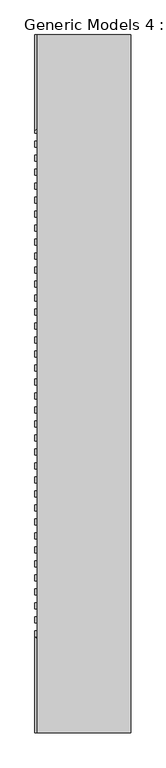
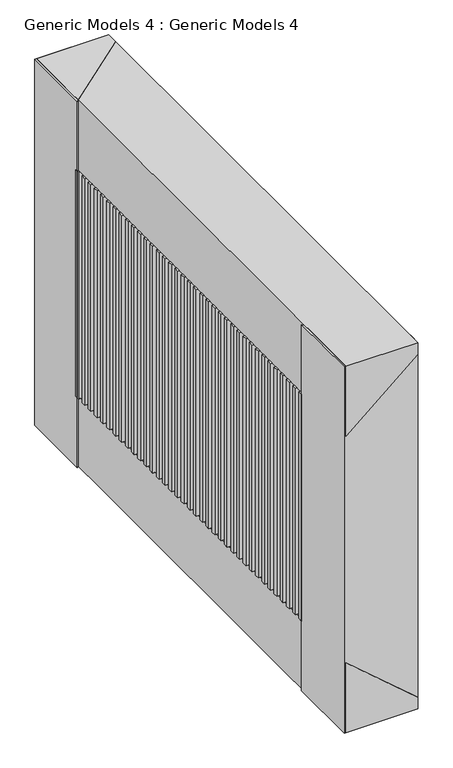
"""IFC4 building model written with IfcOpenShell, lengths in millimetres: proxy geometry, Generic Models 4 : Generic Models 4."""

from ifc_helpers import new_model, si_unit, frame, origin, place, context, project, spatial, polyline, outline, extrude, source, transform, mapped, element, save


def generic_models_4_generic_models_4_3dac0b09(model_context):
    return source(origin(), model_context, "Body", "SweptSolid", [
        extrude(outline(polyline([(7553.0590234, -3519.1296941), (7591.1590234, -3519.1296941), (7591.1590234, -3557.2296941), (7553.0590234, -3557.2296941), (7553.0590234, -3519.1296941)])), frame((0.0, 0.0, 4114.8), z_axis=(0.0, 0.0, 1.0), x_axis=(1.0, 0.0, 0.0)), (0.0, 0.0, 1.0), 1981.2),
        extrude(outline(polyline([(7553.0590234, -3430.2296941), (7591.1590234, -3430.2296941), (7591.1590234, -3468.3296941), (7553.0590234, -3468.3296941), (7553.0590234, -3430.2296941)])), frame((0.0, 0.0, 4114.8), z_axis=(0.0, 0.0, 1.0), x_axis=(1.0, 0.0, 0.0)), (0.0, 0.0, 1.0), 1981.2),
        extrude(outline(polyline([(7553.0590234, -3341.3296941), (7591.1590234, -3341.3296941), (7591.1590234, -3379.4296941), (7553.0590234, -3379.4296941), (7553.0590234, -3341.3296941)])), frame((0.0, 0.0, 4114.8), z_axis=(0.0, 0.0, 1.0), x_axis=(1.0, 0.0, 0.0)), (0.0, 0.0, 1.0), 1981.2),
        extrude(outline(polyline([(7553.0590234, -3252.4296941), (7591.1590234, -3252.4296941), (7591.1590234, -3290.5296941), (7553.0590234, -3290.5296941), (7553.0590234, -3252.4296941)])), frame((0.0, 0.0, 4114.8), z_axis=(0.0, 0.0, 1.0), x_axis=(1.0, 0.0, 0.0)), (0.0, 0.0, 1.0), 1981.2),
        extrude(outline(polyline([(7553.0590234, -3163.5296941), (7591.1590234, -3163.5296941), (7591.1590234, -3201.6296941), (7553.0590234, -3201.6296941), (7553.0590234, -3163.5296941)])), frame((0.0, 0.0, 4114.8), z_axis=(0.0, 0.0, 1.0), x_axis=(1.0, 0.0, 0.0)), (0.0, 0.0, 1.0), 1981.2),
        extrude(outline(polyline([(7553.0590234, -3074.6296941), (7591.1590234, -3074.6296941), (7591.1590234, -3112.7296941), (7553.0590234, -3112.7296941), (7553.0590234, -3074.6296941)])), frame((0.0, 0.0, 4114.8), z_axis=(0.0, 0.0, 1.0), x_axis=(1.0, 0.0, 0.0)), (0.0, 0.0, 1.0), 1981.2),
        extrude(outline(polyline([(7553.0590234, -2985.7296941), (7591.1590234, -2985.7296941), (7591.1590234, -3023.8296941), (7553.0590234, -3023.8296941), (7553.0590234, -2985.7296941)])), frame((0.0, 0.0, 4114.8), z_axis=(0.0, 0.0, 1.0), x_axis=(1.0, 0.0, 0.0)), (0.0, 0.0, 1.0), 1981.2),
        extrude(outline(polyline([(7553.0590234, -2896.8296941), (7591.1590234, -2896.8296941), (7591.1590234, -2934.9296941), (7553.0590234, -2934.9296941), (7553.0590234, -2896.8296941)])), frame((0.0, 0.0, 4114.8), z_axis=(0.0, 0.0, 1.0), x_axis=(1.0, 0.0, 0.0)), (0.0, 0.0, 1.0), 1981.2),
        extrude(outline(polyline([(7553.0590234, -2807.9296941), (7591.1590234, -2807.9296941), (7591.1590234, -2846.0296941), (7553.0590234, -2846.0296941), (7553.0590234, -2807.9296941)])), frame((0.0, 0.0, 4114.8), z_axis=(0.0, 0.0, 1.0), x_axis=(1.0, 0.0, 0.0)), (0.0, 0.0, 1.0), 1981.2),
        extrude(outline(polyline([(7553.0590234, -2719.0296941), (7591.1590234, -2719.0296941), (7591.1590234, -2757.1296941), (7553.0590234, -2757.1296941), (7553.0590234, -2719.0296941)])), frame((0.0, 0.0, 4114.8), z_axis=(0.0, 0.0, 1.0), x_axis=(1.0, 0.0, 0.0)), (0.0, 0.0, 1.0), 1981.2),
        extrude(outline(polyline([(7553.0590234, -2630.1296941), (7591.1590234, -2630.1296941), (7591.1590234, -2668.2296941), (7553.0590234, -2668.2296941), (7553.0590234, -2630.1296941)])), frame((0.0, 0.0, 4114.8), z_axis=(0.0, 0.0, 1.0), x_axis=(1.0, 0.0, 0.0)), (0.0, 0.0, 1.0), 1981.2),
        extrude(outline(polyline([(7553.0590234, -2541.2296941), (7591.1590234, -2541.2296941), (7591.1590234, -2579.3296941), (7553.0590234, -2579.3296941), (7553.0590234, -2541.2296941)])), frame((0.0, 0.0, 4114.8), z_axis=(0.0, 0.0, 1.0), x_axis=(1.0, 0.0, 0.0)), (0.0, 0.0, 1.0), 1981.2),
        extrude(outline(polyline([(7553.0590234, -2452.3296941), (7591.1590234, -2452.3296941), (7591.1590234, -2490.4296941), (7553.0590234, -2490.4296941), (7553.0590234, -2452.3296941)])), frame((0.0, 0.0, 4114.8), z_axis=(0.0, 0.0, 1.0), x_axis=(1.0, 0.0, 0.0)), (0.0, 0.0, 1.0), 1981.2),
        extrude(outline(polyline([(7553.0590234, -2363.4296941), (7591.1590234, -2363.4296941), (7591.1590234, -2401.5296941), (7553.0590234, -2401.5296941), (7553.0590234, -2363.4296941)])), frame((0.0, 0.0, 4114.8), z_axis=(0.0, 0.0, 1.0), x_axis=(1.0, 0.0, 0.0)), (0.0, 0.0, 1.0), 1981.2),
        extrude(outline(polyline([(7553.0590234, -2274.5296941), (7591.1590234, -2274.5296941), (7591.1590234, -2312.6296941), (7553.0590234, -2312.6296941), (7553.0590234, -2274.5296941)])), frame((0.0, 0.0, 4114.8), z_axis=(0.0, 0.0, 1.0), x_axis=(1.0, 0.0, 0.0)), (0.0, 0.0, 1.0), 1981.2),
        extrude(outline(polyline([(7553.0590234, -2185.6296941), (7591.1590234, -2185.6296941), (7591.1590234, -2223.7296941), (7553.0590234, -2223.7296941), (7553.0590234, -2185.6296941)])), frame((0.0, 0.0, 4114.8), z_axis=(0.0, 0.0, 1.0), x_axis=(1.0, 0.0, 0.0)), (0.0, 0.0, 1.0), 1981.2),
        extrude(outline(polyline([(7553.0590234, -2096.7296941), (7591.1590234, -2096.7296941), (7591.1590234, -2134.8296941), (7553.0590234, -2134.8296941), (7553.0590234, -2096.7296941)])), frame((0.0, 0.0, 4114.8), z_axis=(0.0, 0.0, 1.0), x_axis=(1.0, 0.0, 0.0)), (0.0, 0.0, 1.0), 1981.2),
        extrude(outline(polyline([(7553.0590234, -2007.8296941), (7591.1590234, -2007.8296941), (7591.1590234, -2045.9296941), (7553.0590234, -2045.9296941), (7553.0590234, -2007.8296941)])), frame((0.0, 0.0, 4114.8), z_axis=(0.0, 0.0, 1.0), x_axis=(1.0, 0.0, 0.0)), (0.0, 0.0, 1.0), 1981.2),
        extrude(outline(polyline([(7553.0590234, -1918.9296941), (7591.1590234, -1918.9296941), (7591.1590234, -1957.0296941), (7553.0590234, -1957.0296941), (7553.0590234, -1918.9296941)])), frame((0.0, 0.0, 4114.8), z_axis=(0.0, 0.0, 1.0), x_axis=(1.0, 0.0, 0.0)), (0.0, 0.0, 1.0), 1981.2),
        extrude(outline(polyline([(7553.0590234, -1830.0296941), (7591.1590234, -1830.0296941), (7591.1590234, -1868.1296941), (7553.0590234, -1868.1296941), (7553.0590234, -1830.0296941)])), frame((0.0, 0.0, 4114.8), z_axis=(0.0, 0.0, 1.0), x_axis=(1.0, 0.0, 0.0)), (0.0, 0.0, 1.0), 1981.2),
        extrude(outline(polyline([(7553.0590234, -1741.1296941), (7591.1590234, -1741.1296941), (7591.1590234, -1779.2296941), (7553.0590234, -1779.2296941), (7553.0590234, -1741.1296941)])), frame((0.0, 0.0, 4114.8), z_axis=(0.0, 0.0, 1.0), x_axis=(1.0, 0.0, 0.0)), (0.0, 0.0, 1.0), 1981.2),
        extrude(outline(polyline([(7553.0590234, -1652.2296941), (7591.1590234, -1652.2296941), (7591.1590234, -1690.3296941), (7553.0590234, -1690.3296941), (7553.0590234, -1652.2296941)])), frame((0.0, 0.0, 4114.8), z_axis=(0.0, 0.0, 1.0), x_axis=(1.0, 0.0, 0.0)), (0.0, 0.0, 1.0), 1981.2),
        extrude(outline(polyline([(7553.0590234, -1563.3296941), (7591.1590234, -1563.3296941), (7591.1590234, -1601.4296941), (7553.0590234, -1601.4296941), (7553.0590234, -1563.3296941)])), frame((0.0, 0.0, 4114.8), z_axis=(0.0, 0.0, 1.0), x_axis=(1.0, 0.0, 0.0)), (0.0, 0.0, 1.0), 1981.2),
        extrude(outline(polyline([(7553.0590234, -1474.4296941), (7591.1590234, -1474.4296941), (7591.1590234, -1512.5296941), (7553.0590234, -1512.5296941), (7553.0590234, -1474.4296941)])), frame((0.0, 0.0, 4114.8), z_axis=(0.0, 0.0, 1.0), x_axis=(1.0, 0.0, 0.0)), (0.0, 0.0, 1.0), 1981.2),
        extrude(outline(polyline([(7553.0590234, -1385.5296941), (7591.1590234, -1385.5296941), (7591.1590234, -1423.6296941), (7553.0590234, -1423.6296941), (7553.0590234, -1385.5296941)])), frame((0.0, 0.0, 4114.8), z_axis=(0.0, 0.0, 1.0), x_axis=(1.0, 0.0, 0.0)), (0.0, 0.0, 1.0), 1981.2),
        extrude(outline(polyline([(7553.0590234, -1296.6296941), (7591.1590234, -1296.6296941), (7591.1590234, -1334.7296941), (7553.0590234, -1334.7296941), (7553.0590234, -1296.6296941)])), frame((0.0, 0.0, 4114.8), z_axis=(0.0, 0.0, 1.0), x_axis=(1.0, 0.0, 0.0)), (0.0, 0.0, 1.0), 1981.2),
        extrude(outline(polyline([(7553.0590234, -1207.7296941), (7591.1590234, -1207.7296941), (7591.1590234, -1245.8296941), (7553.0590234, -1245.8296941), (7553.0590234, -1207.7296941)])), frame((0.0, 0.0, 4114.8), z_axis=(0.0, 0.0, 1.0), x_axis=(1.0, 0.0, 0.0)), (0.0, 0.0, 1.0), 1981.2),
        extrude(outline(polyline([(7553.0590234, -1118.8296941), (7591.1590234, -1118.8296941), (7591.1590234, -1156.9296941), (7553.0590234, -1156.9296941), (7553.0590234, -1118.8296941)])), frame((0.0, 0.0, 4114.8), z_axis=(0.0, 0.0, 1.0), x_axis=(1.0, 0.0, 0.0)), (0.0, 0.0, 1.0), 1981.2),
        extrude(outline(polyline([(7553.0590234, -1029.9296941), (7591.1590234, -1029.9296941), (7591.1590234, -1068.0296941), (7553.0590234, -1068.0296941), (7553.0590234, -1029.9296941)])), frame((0.0, 0.0, 4114.8), z_axis=(0.0, 0.0, 1.0), x_axis=(1.0, 0.0, 0.0)), (0.0, 0.0, 1.0), 1981.2),
        extrude(outline(polyline([(7553.0590234, -941.0296941), (7591.1590234, -941.0296941), (7591.1590234, -979.1296941), (7553.0590234, -979.1296941), (7553.0590234, -941.0296941)])), frame((0.0, 0.0, 4114.8), z_axis=(0.0, 0.0, 1.0), x_axis=(1.0, 0.0, 0.0)), (0.0, 0.0, 1.0), 1981.2),
        extrude(outline(polyline([(7553.0590234, -852.1296941), (7591.1590234, -852.1296941), (7591.1590234, -890.2296941), (7553.0590234, -890.2296941), (7553.0590234, -852.1296941)])), frame((0.0, 0.0, 4114.8), z_axis=(0.0, 0.0, 1.0), x_axis=(1.0, 0.0, 0.0)), (0.0, 0.0, 1.0), 1981.2),
        extrude(outline(polyline([(7553.0590234, -763.2296941), (7591.1590234, -763.2296941), (7591.1590234, -801.3296941), (7553.0590234, -801.3296941), (7553.0590234, -763.2296941)])), frame((0.0, 0.0, 4114.8), z_axis=(0.0, 0.0, 1.0), x_axis=(1.0, 0.0, 0.0)), (0.0, 0.0, 1.0), 1981.2),
        extrude(outline(polyline([(7553.0590234, -674.3296941), (7591.1590234, -674.3296941), (7591.1590234, -712.4296941), (7553.0590234, -712.4296941), (7553.0590234, -674.3296941)])), frame((0.0, 0.0, 4114.8), z_axis=(0.0, 0.0, 1.0), x_axis=(1.0, 0.0, 0.0)), (0.0, 0.0, 1.0), 1981.2),
        extrude(outline(polyline([(7553.0590234, -585.4296941), (7591.1590234, -585.4296941), (7591.1590234, -623.5296941), (7553.0590234, -623.5296941), (7553.0590234, -585.4296941)])), frame((0.0, 0.0, 4114.8), z_axis=(0.0, 0.0, 1.0), x_axis=(1.0, 0.0, 0.0)), (0.0, 0.0, 1.0), 1981.2),
        extrude(outline(polyline([(7553.0590234, -496.5296941), (7591.1590234, -496.5296941), (7591.1590234, -534.6296941), (7553.0590234, -534.6296941), (7553.0590234, -496.5296941)])), frame((0.0, 0.0, 4114.8), z_axis=(0.0, 0.0, 1.0), x_axis=(1.0, 0.0, 0.0)), (0.0, 0.0, 1.0), 1981.2),
        extrude(outline(polyline([(7553.0590234, -407.6296941), (7591.1590234, -407.6296941), (7591.1590234, -445.7296941), (7553.0590234, -445.7296941), (7553.0590234, -407.6296941)])), frame((0.0, 0.0, 4114.8), z_axis=(0.0, 0.0, 1.0), x_axis=(1.0, 0.0, 0.0)), (0.0, 0.0, 1.0), 1981.2),
        extrude(outline(polyline([(7553.0590234, -318.7296941), (7591.1590234, -318.7296941), (7591.1590234, -356.8296941), (7553.0590234, -356.8296941), (7553.0590234, -318.7296941)])), frame((0.0, 0.0, 4114.8), z_axis=(0.0, 0.0, 1.0), x_axis=(1.0, 0.0, 0.0)), (0.0, 0.0, 1.0), 1981.2),
        extrude(outline(polyline([(3505.2, 8162.6590234), (3606.8, 8162.6590234), (4114.8, 7567.1057451), (3505.2, 7567.1057451), (3505.2, 8162.6590234)])), frame((0.0, -4166.8296941, 0.0), z_axis=(0.0, 1.0, 0.0), x_axis=(0.0, 0.0, 1.0)), (0.0, 0.0, 1.0), 4434.2439479),
        extrude(outline(polyline([(6705.6, 8162.6590234), (6705.6, 7567.1057451), (6096.0, 7567.1057451), (6604.0, 8162.6590234), (6705.6, 8162.6590234)])), frame((0.0, -4166.8296941, 0.0), z_axis=(0.0, 1.0, 0.0), x_axis=(0.0, 0.0, 1.0)), (0.0, 0.0, 1.0), 4434.2439479),
        extrude(outline(polyline([(7553.0590234, -3557.2296941), (8162.6590234, -4065.2296941), (8162.6590234, -4166.8296941), (7553.0590234, -4166.8296941), (7553.0590234, -3557.2296941)])), frame((0.0, 0.0, 3505.2), z_axis=(0.0, 0.0, 1.0), x_axis=(1.0, 0.0, 0.0)), (0.0, 0.0, 1.0), 3200.4),
        extrude(outline(polyline([(7553.0590234, -342.1857463), (7553.0590234, 267.4142537), (8162.6590234, 267.4142537), (8162.6590234, 165.8142537), (7553.0590234, -342.1857463)])), frame((0.0, 0.0, 3505.2), z_axis=(0.0, 0.0, 1.0), x_axis=(1.0, 0.0, 0.0)), (0.0, 0.0, 1.0), 3200.4),
    ])


if __name__ == "__main__":
    model = new_model("IFC4")
    model_context = context("Model", 3, world=origin())
    ifc_project = project(units=[si_unit("LENGTHUNIT", "METRE", prefix="MILLI")], contexts=[model_context])
    site = spatial("IfcSite", under=ifc_project)
    building = spatial("IfcBuilding", under=site)
    placement = place(None, origin())
    generic_models_4_generic_models_4_shape = generic_models_4_generic_models_4_3dac0b09(model_context)
    element("IfcBuildingElementProxy", 1, Name="Generic Models 4 : Generic Models 4", ObjectType="Generic Models 4 : Generic Models 4", at=placement, inside=building, context=model_context, shape_type="MappedRepresentation", body=[
        mapped(generic_models_4_generic_models_4_shape, transform((0.0, 0.0, 0.0), x_axis=(1.0, 0.0, 0.0), y_axis=(0.0, 1.0, 0.0), z_axis=(0.0, 0.0, 1.0))),
    ])
    save(model, "model.ifc")

# Revit data of these elements
# Element 1 (IfcBuildingElementProxy, "Generic Models 4 : Generic Models 4")
#   Materials on its faces: "Default New Material"
# Materials
#   "Default New Material": class "Generic", colour RGB 64 128 128, transparency 0, Cost = 0
